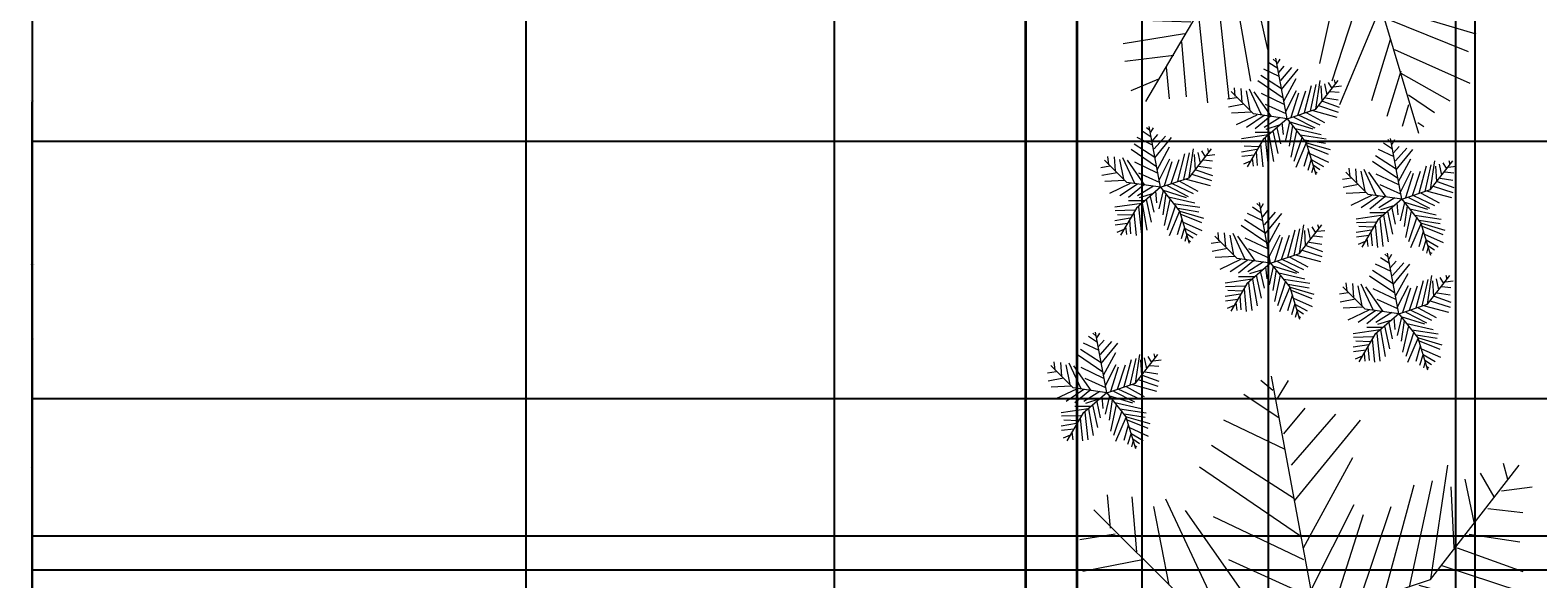
# Model space of a CAD drawing. Units: inches. Extents: x 818 to 1898, y 976 to 2364.
# Tile 60 of 96: x 818 to 1083, y 2046 to 2142. Entities that reach past the tile are written whole.
import ezdxf

# ---------------------------------------------------------------- set-up
doc = ezdxf.new("R2010")
doc.units = ezdxf.units.IN
doc.header["$LTSCALE"] = 5
doc.header["$MEASUREMENT"] = 0
for name, color, linetype, lineweight in [('A-ANNO-DIMS', 2, 'Continuous', 18), ('C-PROP', 7, 'Continuous', 35), ('L-PLNT-BEDS', 94, 'Continuous', 18)]:
    doc.layers.add(name, color=color, linetype=linetype, lineweight=lineweight)
doc.layers.add('L-PLNT', color=116, linetype='Continuous', lineweight=13, true_color=0x136734)
doc.styles.get("Standard").update_dxf_attribs({"font": 'arial.ttf'})
doc.dimstyles.get("Standard").update_dxf_attribs({"dimtxt": 0.18, "dimasz": 0.18, "dimexe": 0.18, "dimexo": 0.0625, "dimgap": 0.09, "dimtad": 0, "dimtih": 1, "dimtoh": 1, "dimdec": 4, "dimzin": 0, "dimdsep": 46, "dimtxsty": 'Standard', "dimcen": 0.09, "dimadec": 0, "dimazin": 0, "dimtfac": 1, "dimtdec": 4, "dimtofl": 0, "dimtmove": 0, "dimatfit": 3, "dimfxl": 1, "dimtolj": 1, "dimtzin": 0, "dimarcsym": 0})

# ---------------------------------------------------------------- blocks, each defined once
blk = doc.blocks.new('SHRUB-ACCENT')
for p, q in [((8.8, 18.63), (7.25, 19.67)), ((8.53, 19.84), (7.99, 20.28)), ((10.44, 9.82), (8.47, 20.47)), ((8.74, 19.5), (9.21, 20.28)), ((9.01, 17.93), (9.96, 19.06)), ((9.35, 16.54), (11.31, 18.8)), ((9.75, 13.42), (5.28, 16.46)), ((9.48, 15.07), (5.82, 17.41)), ((9.08, 17.24), (6.37, 18.54)), ((9.48, 14.98), (12.39, 18.54)), ((9.89, 12.9), (12.06, 16.89)), ((15.49, 11.5), (19.41, 16.55)), ((15.51, 11.51), (16.25, 16.54)), ((17, 15.94), (17.41, 14.03)), ((17.68, 16.2), (18.29, 15.16)), ((18.69, 16.63), (18.9, 15.94)), ((1.56, 13.51), (0, 13.25)), ((4.55, 10.66), (0.62, 14.58)), ((1.35, 13.77), (1.22, 15.24)), ((2.3, 15.16), (2.51, 12.72)), ((3.25, 14.72), (3.93, 11.25)), ((3.79, 15.07), (5.89, 10.55)), ((7.72, 10.21), (4.67, 14.55)), ((5.89, 14.29), (9.89, 12.38)), ((10.23, 11.07), (12.12, 14.81)), ((11.17, 10.12), (12.53, 14.37)), ((12.33, 10.47), (13.75, 14.72)), ((13.48, 10.9), (14.76, 15.68)), ((14.56, 11.16), (15.58, 15.85)), ((16.39, 15.59), (16.53, 12.9)), ((17.2, 13.51), (19.44, 13.16)), ((18.02, 14.63), (19.57, 14.46)), ((18.62, 15.42), (19.98, 15.59)), ((2.84, 12.38), (0.14, 11.86)), ((4.2, 10.99), (0.68, 10.81)), ((10.44, 9.82), (4.55, 10.66)), ((6.57, 12.38), (10.23, 10.73)), ((10.44, 9.82), (15.49, 11.5)), ((13.82, 10.9), (17, 9.16)), ((14.97, 11.25), (19.17, 10.12)), ((15.98, 12.12), (19.44, 10.99)), ((16.66, 12.9), (19.57, 11.86)), ((5.15, 10.47), (1.49, 8.73)), ((6.43, 10.38), (3.32, 8.3)), ((7.45, 10.21), (4.81, 8.04)), ((10.44, 9.82), (6.23, 6.17)), ((9.21, 10.03), (6.43, 8.3)), ((9.21, 8.73), (6.7, 7.95)), ((8.67, 8.21), (9.28, 5.43)), ((9.55, 9.16), (9.75, 7.08)), ((10.9, 9.25), (10.16, 6.04)), ((10.44, 9.82), (13.8, 5.61)), ((10.77, 9.34), (14.97, 8.04)), ((11.38, 8.64), (10.84, 5)), ((11.65, 10.12), (15.31, 8.21)), ((11.85, 8.12), (16.46, 7.08)), ((12.53, 10.47), (16.19, 8.73)), ((7.18, 6.99), (2.44, 6.3)), ((5.89, 5.78), (2.51, 5.69)), ((6.23, 6.17), (3.43, 1.4)), ((7.59, 7.43), (4.81, 7.43)), ((5.76, 5.34), (6.16, 1.35)), ((6.57, 6.39), (7.11, 1.52)), ((7.25, 6.99), (8.06, 2.31)), ((7.92, 7.69), (8.8, 3.69)), ((12.12, 7.69), (11.11, 3.09)), ((13.07, 6.65), (11.65, 2.31)), ((13.82, 5.6), (11.99, 1.26)), ((12.73, 6.99), (17.34, 6.3)), ((13.48, 6.13), (17.2, 5.52)), ((13.8, 5.61), (15.49, 0)), ((13.88, 5.6), (18.02, 4.39)), ((5.15, 4.39), (2.44, 3.95)), ((4.67, 3.43), (2.51, 3.17)), ((5.42, 4.91), (2.91, 5)), ((4.33, 2.91), (4.47, 1.52)), ((5.01, 4.04), (5.21, 1.61)), ((14.22, 4.13), (13.41, 1.44)), ((14.02, 5.08), (17.68, 3.61)), ((14.7, 2.74), (14.09, 0.74)), ((14.43, 3.69), (17.74, 2.22)), ((14.7, 2.65), (16.86, 1.44)), ((4, 2.39), (2.78, 1.87)), ((15.04, 1.26), (14.76, 0.31)), ((15.04, 1.7), (16.19, 0.92)), ((15.44, 0.48), (15.71, 0.31))]:
    blk.add_line(p, q)
blk = doc.blocks.new('PALM-BORDER')
for p, q in [((33.95, 78.95), (31.8, 80.68)), ((41.53, 39.05), (33.72, 81.45)), ((34.76, 77.57), (36.65, 80.68)), ((35.03, 74.11), (28.83, 78.26)), ((35.84, 71.35), (39.61, 75.84)), ((37.18, 65.82), (45, 74.8)), ((36.11, 68.59), (25.33, 73.77)), ((37.72, 59.6), (49.31, 73.77)), ((37.72, 59.95), (23.17, 69.28)), ((39.34, 51.31), (47.96, 67.2)), ((38.8, 53.39), (21.02, 65.48)), ((61.61, 45.75), (77.23, 65.83)), ((61.71, 45.79), (64.67, 65.82)), ((70.33, 64.44), (72.75, 60.3)), ((74.37, 66.17), (75.18, 63.4)), ((53.62, 43.37), (58.74, 62.37)), ((57.93, 44.41), (61.97, 63.06)), ((65.21, 62.02), (65.75, 51.31)), ((67.63, 63.4), (69.25, 55.81)), ((74.1, 61.33), (79.49, 62.02)), ((5.39, 54.77), (4.85, 60.64)), ((9.16, 60.3), (9.97, 50.62)), ((12.93, 58.57), (15.63, 44.75)), ((15.09, 59.95), (23.44, 41.99)), ((40.69, 44.06), (48.23, 58.91)), ((49.04, 41.64), (54.7, 58.57)), ((18.1, 42.4), (2.48, 58.02)), ((30.72, 40.61), (18.59, 57.88)), ((23.44, 56.84), (39.34, 49.24)), ((44.46, 40.26), (49.85, 57.19)), ((71.68, 58.22), (77.87, 57.53)), ((6.2, 53.73), (0, 52.7)), ((68.44, 53.73), (77.33, 52.35)), ((66.29, 51.31), (77.87, 47.17)), ((11.32, 49.24), (0.54, 47.17)), ((26.14, 49.24), (40.69, 42.68)), ((63.59, 48.21), (77.33, 43.71)), ((41.53, 39.05), (61.61, 45.75)), ((16.71, 43.71), (2.69, 43.02)), ((41.53, 39.05), (18.1, 42.4)), ((54.97, 43.37), (67.63, 36.46)), ((59.55, 44.75), (76.26, 40.26)), ((20.48, 41.64), (5.93, 34.73)), ((25.6, 41.3), (13.2, 33.01)), ((29.64, 40.61), (19.13, 31.97)), ((36.65, 39.91), (25.6, 33.01)), ((46.35, 40.26), (60.9, 32.66)), ((49.85, 41.64), (64.4, 34.73)), ((41.53, 39.05), (24.79, 24.55)), ((41.53, 39.05), (54.92, 22.32)), ((42.84, 37.15), (59.55, 31.97)), ((36.65, 34.73), (26.68, 31.62)), ((37.99, 36.46), (38.8, 28.17)), ((43.38, 36.81), (40.42, 24.02)), ((34.49, 32.66), (36.92, 21.61)), ((45.27, 34.39), (43.11, 19.88)), ((47.15, 32.32), (65.48, 28.17)), ((30.18, 29.55), (19.13, 29.55)), ((31.53, 30.59), (35.03, 14.7)), ((48.23, 30.59), (44.19, 12.28)), ((28.56, 27.82), (9.7, 25.06)), ((28.83, 27.82), (32.07, 9.17)), ((50.66, 27.82), (68.98, 25.06)), ((24.79, 24.55), (13.63, 5.58)), ((26.14, 25.41), (28.29, 6.06)), ((52, 26.44), (46.35, 9.17)), ((53.62, 24.37), (68.44, 21.95)), ((23.44, 22.99), (9.97, 22.64)), ((22.9, 21.26), (24.52, 5.37)), ((54.97, 22.3), (47.69, 5.02)), ((54.92, 22.32), (61.61, 0)), ((55.24, 22.3), (71.68, 17.46)), ((21.56, 19.53), (11.59, 19.88)), ((55.78, 20.22), (70.33, 14.35)), ((20.48, 17.46), (9.7, 15.73)), ((19.94, 16.08), (20.75, 6.41)), ((56.59, 16.42), (53.35, 5.72)), ((18.59, 13.66), (9.97, 12.62)), ((57.39, 14.7), (70.6, 8.83)), ((17.24, 11.59), (17.78, 6.06)), ((58.47, 10.9), (56.05, 2.95)), ((15.9, 9.52), (11.05, 7.44)), ((58.47, 10.55), (67.09, 5.72)), ((59.82, 6.75), (64.4, 3.64)), ((59.82, 5.02), (58.74, 1.22)), ((61.44, 1.92), (62.51, 1.22))]:
    blk.add_line(p, q)
blk = doc.blocks.new('PALM-DECK')
for p, q in [((60.66, 141.05), (56.81, 144.14)), ((74.19, 69.77), (60.24, 145.52)), ((62.1, 138.58), (65.47, 144.14)), ((62.58, 132.41), (51.51, 139.82)), ((64.03, 127.47), (70.77, 135.5)), ((66.43, 117.6), (80.4, 133.65)), ((64.51, 122.54), (45.25, 131.79)), ((67.4, 106.49), (88.1, 131.79)), ((67.4, 107.11), (41.4, 123.77)), ((70.29, 91.68), (85.69, 120.07)), ((69.32, 95.38), (37.55, 116.98)), ((110.08, 81.73), (137.98, 117.61)), ((110.24, 81.8), (115.54, 117.6)), ((132.87, 118.22), (134.31, 113.28)), ((125.65, 115.13), (129.98, 107.72)), ((95.8, 77.48), (104.95, 111.43)), ((103.5, 79.33), (110.72, 112.66)), ((120.83, 113.28), (123.72, 99.7)), ((116.5, 110.81), (117.47, 91.68)), ((132.39, 109.58), (142.02, 110.81)), ((9.63, 97.85), (8.67, 108.34)), ((16.37, 107.72), (17.81, 90.44)), ((26.96, 107.11), (41.88, 75.01)), ((32.33, 75.75), (4.43, 103.66)), ((23.11, 104.64), (27.92, 79.95)), ((54.88, 72.55), (33.22, 103.4)), ((72.69, 78.72), (86.17, 105.26)), ((87.62, 74.4), (97.73, 104.64)), ((128.06, 104.02), (139.13, 102.79)), ((41.88, 101.55), (70.29, 87.97)), ((79.43, 71.93), (89.06, 102.17)), ((11.07, 96), (0, 94.15)), ((122.28, 96), (138.16, 93.53)), ((118.43, 91.68), (139.13, 84.27)), ((20.22, 87.97), (0.96, 84.27)), ((46.7, 87.97), (72.69, 76.25)), ((113.61, 86.12), (138.16, 78.1)), ((74.19, 69.77), (110.08, 81.73)), ((106.39, 79.95), (136.24, 71.93)), ((29.85, 78.1), (4.81, 76.87)), ((98.21, 77.48), (120.83, 65.14)), ((36.59, 74.4), (10.59, 62.05)), ((74.19, 69.77), (32.33, 75.75)), ((89.06, 74.4), (115.06, 62.05)), ((45.73, 73.78), (23.59, 58.97)), ((52.96, 72.55), (34.18, 57.12)), ((82.8, 71.93), (108.8, 58.35)), ((74.19, 69.77), (44.29, 43.85)), ((65.47, 71.31), (45.73, 58.97)), ((74.19, 69.77), (98.11, 39.87)), ((76.54, 66.37), (106.39, 57.12)), ((67.88, 65.14), (69.32, 50.33)), ((77.51, 65.76), (72.21, 42.92)), ((65.47, 62.05), (47.66, 56.5)), ((80.88, 61.44), (77.03, 35.52)), ((61.62, 58.35), (65.95, 38.6)), ((84.25, 57.73), (116.98, 50.33)), ((56.33, 54.65), (62.58, 26.26)), ((86.17, 54.65), (78.95, 21.94)), ((53.92, 52.8), (34.18, 52.8)), ((51.03, 49.71), (17.33, 44.77)), ((51.51, 49.71), (57.29, 16.38)), ((90.51, 49.71), (123.24, 44.77)), ((46.7, 45.39), (50.55, 10.83)), ((92.91, 47.24), (82.8, 16.38)), ((44.29, 43.85), (24.36, 9.97)), ((95.8, 43.54), (122.28, 39.22)), ((41.88, 41.07), (17.81, 40.45)), ((98.21, 39.84), (85.21, 8.98)), ((98.11, 39.87), (110.08, 0)), ((98.69, 39.84), (128.06, 31.2)), ((40.92, 37.98), (43.81, 9.59)), ((38.51, 34.9), (20.7, 35.52)), ((99.65, 36.13), (125.65, 25.64)), ((36.59, 31.2), (17.33, 28.11)), ((101.1, 29.34), (95.32, 10.21)), ((35.62, 28.73), (37.07, 11.45)), ((33.22, 24.41), (17.81, 22.55)), ((102.54, 26.26), (126.13, 15.77)), ((30.81, 20.7), (31.77, 10.83)), ((104.47, 19.47), (100.13, 5.27)), ((104.47, 18.85), (119.87, 10.21)), ((28.4, 17), (19.74, 13.3)), ((106.87, 12.06), (115.06, 6.51)), ((106.87, 8.98), (104.95, 2.19)), ((109.76, 3.42), (111.69, 2.19))]:
    blk.add_line(p, q)
blk = doc.blocks.new('*D59')
at = {"layer": 'A-ANNO-DIMS', "color": 0, "lineweight": -2, "ltscale": 5, "transparency": 16777216}
for p, q in [((1251.64, 2300.39), (818.03, 2300.39)), ((818.21, 2300.21), (818.21, 1669.95)), ((818.21, 1039.32), (818.21, 1669.59)), ((896.05, 1039.14), (818.03, 1039.14))]:
    blk.add_line(p, q, dxfattribs=at)
at = {"layer": 'A-ANNO-DIMS', "color": 0, "ltscale": 5, "transparency": 16777216}
for points in [[(818.18, 2300.21), (818.24, 2300.21), (818.21, 2300.39)], [(818.18, 1039.32), (818.24, 1039.32), (818.21, 1039.14)]]:
    blk.add_solid(points, dxfattribs=at)
at = {"layer": 'Defpoints', "color": 0, "ltscale": 5, "transparency": 16777216}
for p in [(818.21, 2300.39), (1251.71, 2300.39), (896.11, 1039.14)]:
    blk.add_point(p, dxfattribs=at)
at = {"layer": 'A-ANNO-DIMS', "color": 0, "ltscale": 5, "transparency": 16777216, "insert": (818.21, 1669.77), "char_height": 0.18, "attachment_point": 5}
blk.add_mtext('\\A1;1261.2', dxfattribs=at)
blk = doc.blocks.new('*D60')
at = {"layer": 'A-ANNO-DIMS', "color": 0, "lineweight": -2, "ltscale": 5, "transparency": 16777216}
for p, q in [((992.66, 2294.22), (818.03, 2294.22)), ((818.21, 2294.04), (818.21, 1748.77)), ((818.21, 1203.14), (818.21, 1748.41)), ((992.66, 1202.96), (818.03, 1202.96))]:
    blk.add_line(p, q, dxfattribs=at)
at = {"layer": 'A-ANNO-DIMS', "color": 0, "ltscale": 5, "transparency": 16777216}
for points in [[(818.18, 2294.04), (818.24, 2294.04), (818.21, 2294.22)], [(818.18, 1203.14), (818.24, 1203.14), (818.21, 1202.96)]]:
    blk.add_solid(points, dxfattribs=at)
at = {"layer": 'Defpoints', "color": 0, "ltscale": 5, "transparency": 16777216}
for p in [(818.21, 2294.22), (992.73, 2294.22), (992.73, 1202.96)]:
    blk.add_point(p, dxfattribs=at)
at = {"layer": 'A-ANNO-DIMS', "color": 0, "ltscale": 5, "transparency": 16777216, "insert": (818.21, 1748.59), "char_height": 0.18, "attachment_point": 5}
blk.add_mtext('\\A1;1091.3', dxfattribs=at)
blk = doc.blocks.new('*D61')
at = {"layer": 'A-ANNO-DIMS', "color": 0, "lineweight": -2, "ltscale": 5, "transparency": 16777216}
for p, q in [((1071.73, 1203.03), (1071.73, 2363.87)), ((1071.91, 2363.69), (1250.94, 2363.69)), ((1430.55, 2363.69), (1251.51, 2363.69)), ((1430.73, 1203.03), (1430.73, 2363.87))]:
    blk.add_line(p, q, dxfattribs=at)
at = {"layer": 'A-ANNO-DIMS', "color": 0, "ltscale": 5, "transparency": 16777216}
for points in [[(1071.91, 2363.72), (1071.91, 2363.66), (1071.73, 2363.69)], [(1430.55, 2363.72), (1430.55, 2363.66), (1430.73, 2363.69)]]:
    blk.add_solid(points, dxfattribs=at)
at = {"layer": 'Defpoints', "color": 0, "ltscale": 5, "transparency": 16777216}
for p in [(1430.73, 2363.69), (1071.73, 1202.96), (1430.73, 1202.96)]:
    blk.add_point(p, dxfattribs=at)
at = {"layer": 'A-ANNO-DIMS', "color": 0, "ltscale": 5, "transparency": 16777216, "insert": (1251.23, 2363.69), "char_height": 0.18, "attachment_point": 5}
blk.add_mtext('\\A1;359', dxfattribs=at)
blk = doc.blocks.new('*D67')
at = {"layer": 'A-ANNO-DIMS', "color": 0, "lineweight": -2, "ltscale": 5, "transparency": 16777216}
for p, q in [((1083.66, 2205.97), (818.03, 2205.97)), ((818.21, 2205.79), (818.21, 2129.71)), ((818.21, 2053.26), (818.21, 2129.34)), ((1083.66, 2053.08), (818.03, 2053.08))]:
    blk.add_line(p, q, dxfattribs=at)
at = {"layer": 'A-ANNO-DIMS', "color": 0, "ltscale": 5, "transparency": 16777216}
for points in [[(818.18, 2205.79), (818.24, 2205.79), (818.21, 2205.97)], [(818.18, 2053.26), (818.24, 2053.26), (818.21, 2053.08)]]:
    blk.add_solid(points, dxfattribs=at)
at = {"layer": 'Defpoints', "color": 0, "ltscale": 5, "transparency": 16777216}
for p in [(818.21, 2205.97), (1083.73, 2205.97), (1083.73, 2053.08)]:
    blk.add_point(p, dxfattribs=at)
at = {"layer": 'A-ANNO-DIMS', "color": 0, "ltscale": 5, "transparency": 16777216, "insert": (818.21, 2129.52), "char_height": 0.18, "attachment_point": 5}
blk.add_mtext('\\A1;152.9', dxfattribs=at)
blk = doc.blocks.new('*D79')
at = {"layer": 'A-ANNO-DIMS', "color": 0, "lineweight": -2, "ltscale": 5, "transparency": 16777216}
for p, q in [((992.73, 1203.03), (992.73, 2363.87)), ((992.91, 2363.69), (1032.01, 2363.69)), ((1071.55, 2363.69), (1032.44, 2363.69)), ((1071.73, 1203.03), (1071.73, 2363.87))]:
    blk.add_line(p, q, dxfattribs=at)
at = {"layer": 'A-ANNO-DIMS', "color": 0, "ltscale": 5, "transparency": 16777216}
for points in [[(992.91, 2363.72), (992.91, 2363.66), (992.73, 2363.69)], [(1071.55, 2363.72), (1071.55, 2363.66), (1071.73, 2363.69)]]:
    blk.add_solid(points, dxfattribs=at)
at = {"layer": 'Defpoints', "color": 0, "ltscale": 5, "transparency": 16777216}
for p in [(1071.73, 2363.69), (992.73, 1202.96), (1071.73, 1202.96)]:
    blk.add_point(p, dxfattribs=at)
at = {"layer": 'A-ANNO-DIMS', "color": 0, "ltscale": 5, "transparency": 16777216, "insert": (1032.23, 2363.69), "char_height": 0.18, "attachment_point": 5}
blk.add_mtext('\\A1;79', dxfattribs=at)
blk = doc.blocks.new('*D90')
at = {"layer": 'A-ANNO-DIMS', "color": 0, "lineweight": -2, "ltscale": 5, "transparency": 16777216}
for p, q in [((904.95, 1071.12), (904.95, 2363.87)), ((905.13, 2363.69), (931.67, 2363.69)), ((958.99, 2363.69), (932.45, 2363.69)), ((959.17, 1071.12), (959.17, 2363.87))]:
    blk.add_line(p, q, dxfattribs=at)
at = {"layer": 'A-ANNO-DIMS', "color": 0, "ltscale": 5, "transparency": 16777216}
for points in [[(905.13, 2363.72), (905.13, 2363.66), (904.95, 2363.69)], [(958.99, 2363.72), (958.99, 2363.66), (959.17, 2363.69)]]:
    blk.add_solid(points, dxfattribs=at)
at = {"layer": 'Defpoints', "color": 0, "ltscale": 5, "transparency": 16777216}
for p in [(959.17, 2363.69), (904.95, 1071.06), (959.17, 1071.06)]:
    blk.add_point(p, dxfattribs=at)
at = {"layer": 'A-ANNO-DIMS', "color": 0, "ltscale": 5, "transparency": 16777216, "insert": (932.06, 2363.69), "char_height": 0.18, "attachment_point": 5}
blk.add_mtext('\\A1;54.22', dxfattribs=at)
blk = doc.blocks.new('*D91')
at = {"layer": 'A-ANNO-DIMS', "color": 0, "lineweight": -2, "ltscale": 5, "transparency": 16777216}
for p, q in [((959.17, 1071.12), (959.17, 2363.87)), ((959.35, 2363.69), (985.8, 2363.69)), ((1013.04, 2363.69), (986.59, 2363.69)), ((1013.22, 1071.12), (1013.22, 2363.87))]:
    blk.add_line(p, q, dxfattribs=at)
at = {"layer": 'A-ANNO-DIMS', "color": 0, "ltscale": 5, "transparency": 16777216}
for points in [[(959.35, 2363.72), (959.35, 2363.66), (959.17, 2363.69)], [(1013.04, 2363.72), (1013.04, 2363.66), (1013.22, 2363.69)]]:
    blk.add_solid(points, dxfattribs=at)
at = {"layer": 'Defpoints', "color": 0, "ltscale": 5, "transparency": 16777216}
for p in [(1013.22, 2363.69), (959.17, 1071.06), (1013.22, 1071.06)]:
    blk.add_point(p, dxfattribs=at)
at = {"layer": 'A-ANNO-DIMS', "color": 0, "ltscale": 5, "transparency": 16777216, "insert": (986.2, 2363.69), "char_height": 0.18, "attachment_point": 5}
blk.add_mtext('\\A1;54.04', dxfattribs=at)
blk = doc.blocks.new('*D92')
at = {"layer": 'A-ANNO-DIMS', "color": 0, "lineweight": -2, "ltscale": 5, "transparency": 16777216}
for p, q in [((1013.22, 1071.12), (1013.22, 2363.87)), ((1013.4, 2363.69), (1040.38, 2363.69)), ((1068.16, 2363.69), (1041.17, 2363.69)), ((1068.34, 1071.12), (1068.34, 2363.87))]:
    blk.add_line(p, q, dxfattribs=at)
at = {"layer": 'A-ANNO-DIMS', "color": 0, "ltscale": 5, "transparency": 16777216}
for points in [[(1013.4, 2363.72), (1013.4, 2363.66), (1013.22, 2363.69)], [(1068.16, 2363.72), (1068.16, 2363.66), (1068.34, 2363.69)]]:
    blk.add_solid(points, dxfattribs=at)
at = {"layer": 'Defpoints', "color": 0, "ltscale": 5, "transparency": 16777216}
for p in [(1068.34, 2363.69), (1013.22, 1071.06), (1068.34, 1071.06)]:
    blk.add_point(p, dxfattribs=at)
at = {"layer": 'A-ANNO-DIMS', "color": 0, "ltscale": 5, "transparency": 16777216, "insert": (1040.78, 2363.69), "char_height": 0.18, "attachment_point": 5}
blk.add_mtext('\\A1;55.12', dxfattribs=at)
blk = doc.blocks.new('*D93')
at = {"layer": 'A-ANNO-DIMS', "color": 0, "lineweight": -2, "ltscale": 5, "transparency": 16777216}
for p, q in [((1068.34, 1071.12), (1068.34, 2363.87)), ((1068.52, 2363.69), (1094.16, 2363.69)), ((1120.58, 2363.69), (1094.94, 2363.69)), ((1120.76, 1071.12), (1120.76, 2363.87))]:
    blk.add_line(p, q, dxfattribs=at)
at = {"layer": 'A-ANNO-DIMS', "color": 0, "ltscale": 5, "transparency": 16777216}
for points in [[(1068.52, 2363.72), (1068.52, 2363.66), (1068.34, 2363.69)], [(1120.58, 2363.72), (1120.58, 2363.66), (1120.76, 2363.69)]]:
    blk.add_solid(points, dxfattribs=at)
at = {"layer": 'Defpoints', "color": 0, "ltscale": 5, "transparency": 16777216}
for p in [(1120.76, 2363.69), (1068.34, 1071.06), (1120.76, 1071.06)]:
    blk.add_point(p, dxfattribs=at)
at = {"layer": 'A-ANNO-DIMS', "color": 0, "ltscale": 5, "transparency": 16777216, "insert": (1094.55, 2363.69), "char_height": 0.18, "attachment_point": 5}
blk.add_mtext('\\A1;52.42', dxfattribs=at)
blk = doc.blocks.new('*D126')
at = {"layer": 'A-ANNO-DIMS', "color": 0, "lineweight": -2, "ltscale": 5, "transparency": 16777216}
for p, q in [((1035.38, 1252.09), (1035.38, 2363.87)), ((1035.56, 2363.69), (1075.41, 2363.69)), ((1116.01, 2363.69), (1076.16, 2363.69)), ((1116.19, 1236.03), (1116.19, 2363.87))]:
    blk.add_line(p, q, dxfattribs=at)
at = {"layer": 'A-ANNO-DIMS', "color": 0, "ltscale": 5, "transparency": 16777216}
for points in [[(1035.56, 2363.72), (1035.56, 2363.66), (1035.38, 2363.69)], [(1116.01, 2363.72), (1116.01, 2363.66), (1116.19, 2363.69)]]:
    blk.add_solid(points, dxfattribs=at)
at = {"layer": 'Defpoints', "color": 0, "ltscale": 5, "transparency": 16777216}
for p in [(1035.38, 2363.69), (1035.38, 1252.02), (1116.19, 1235.96)]:
    blk.add_point(p, dxfattribs=at)
at = {"layer": 'A-ANNO-DIMS', "color": 0, "ltscale": 5, "transparency": 16777216, "insert": (1075.78, 2363.69), "char_height": 0.18, "attachment_point": 5}
blk.add_mtext('\\A1;80.81', dxfattribs=at)
blk = doc.blocks.new('*D133')
at = {"layer": 'A-ANNO-DIMS', "color": 0, "lineweight": -2, "ltscale": 5, "transparency": 16777216}
for p, q in [((1041.64, 2162.89), (818.03, 2162.89)), ((818.21, 2162.71), (818.21, 2101.01)), ((818.21, 2038.94), (818.21, 2100.64)), ((1043.71, 2038.76), (818.03, 2038.76))]:
    blk.add_line(p, q, dxfattribs=at)
at = {"layer": 'A-ANNO-DIMS', "color": 0, "ltscale": 5, "transparency": 16777216}
for points in [[(818.18, 2162.71), (818.24, 2162.71), (818.21, 2162.89)], [(818.18, 2038.94), (818.24, 2038.94), (818.21, 2038.76)]]:
    blk.add_solid(points, dxfattribs=at)
at = {"layer": 'Defpoints', "color": 0, "ltscale": 5, "transparency": 16777216}
for p in [(818.21, 2162.89), (1041.7, 2162.89), (1043.77, 2038.76)]:
    blk.add_point(p, dxfattribs=at)
at = {"layer": 'A-ANNO-DIMS', "color": 0, "ltscale": 5, "transparency": 16777216, "insert": (818.21, 2100.82), "char_height": 0.18, "attachment_point": 5}
blk.add_mtext('\\A1;124.13', dxfattribs=at)
blk = doc.blocks.new('*D146')
at = {"layer": 'A-ANNO-DIMS', "color": 0, "lineweight": -2, "ltscale": 5, "transparency": 16777216}
for p, q in [((1197.33, 2122.38), (818.03, 2122.38)), ((818.21, 2122.2), (818.21, 2087.91)), ((818.21, 2053.26), (818.21, 2087.55)), ((1083.66, 2053.08), (818.03, 2053.08))]:
    blk.add_line(p, q, dxfattribs=at)
at = {"layer": 'A-ANNO-DIMS', "color": 0, "ltscale": 5, "transparency": 16777216}
for points in [[(818.18, 2122.2), (818.24, 2122.2), (818.21, 2122.38)], [(818.18, 2053.26), (818.24, 2053.26), (818.21, 2053.08)]]:
    blk.add_solid(points, dxfattribs=at)
at = {"layer": 'Defpoints', "color": 0, "ltscale": 5, "transparency": 16777216}
for p in [(1197.39, 2122.38), (818.21, 2053.08), (1083.73, 2053.08)]:
    blk.add_point(p, dxfattribs=at)
at = {"layer": 'A-ANNO-DIMS', "color": 0, "ltscale": 5, "transparency": 16777216, "insert": (818.21, 2087.73), "char_height": 0.18, "attachment_point": 5}
blk.add_mtext('\\A1;69.3', dxfattribs=at)
blk = doc.blocks.new('*D257')
at = {"layer": 'A-ANNO-DIMS', "color": 0, "lineweight": -2, "ltscale": 5, "transparency": 16777216}
for p, q in [((1399.57, 2077.19), (818.03, 2077.19)), ((818.21, 2077.01), (818.21, 2065.31)), ((818.21, 2053.26), (818.21, 2064.95)), ((1399.57, 2053.08), (818.03, 2053.08))]:
    blk.add_line(p, q, dxfattribs=at)
at = {"layer": 'A-ANNO-DIMS', "color": 0, "ltscale": 5, "transparency": 16777216}
for points in [[(818.18, 2077.01), (818.24, 2077.01), (818.21, 2077.19)], [(818.18, 2053.26), (818.24, 2053.26), (818.21, 2053.08)]]:
    blk.add_solid(points, dxfattribs=at)
at = {"layer": 'Defpoints', "color": 0, "ltscale": 5, "transparency": 16777216}
for p in [(818.21, 2077.19), (1399.64, 2077.19), (1399.64, 2053.08)]:
    blk.add_point(p, dxfattribs=at)
at = {"layer": 'A-ANNO-DIMS', "color": 0, "ltscale": 5, "transparency": 16777216, "insert": (818.21, 2065.13), "char_height": 0.18, "attachment_point": 5}
blk.add_mtext('\\A1;24.11', dxfattribs=at)
blk = doc.blocks.new('*D266')
at = {"layer": 'A-ANNO-DIMS', "color": 0, "lineweight": -2, "ltscale": 5, "transparency": 16777216}
for p, q in [((1780.44, 2053.08), (818.03, 2053.08)), ((818.21, 2052.9), (818.21, 2050.26)), ((818.21, 2047.26), (818.21, 2049.9)), ((1780.44, 2047.08), (818.03, 2047.08))]:
    blk.add_line(p, q, dxfattribs=at)
at = {"layer": 'A-ANNO-DIMS', "color": 0, "ltscale": 5, "transparency": 16777216}
for points in [[(818.18, 2052.9), (818.24, 2052.9), (818.21, 2053.08)], [(818.18, 2047.26), (818.24, 2047.26), (818.21, 2047.08)]]:
    blk.add_solid(points, dxfattribs=at)
at = {"layer": 'Defpoints', "color": 0, "ltscale": 5, "transparency": 16777216}
for p in [(1780.5, 2053.08), (818.21, 2047.08), (1780.5, 2047.08)]:
    blk.add_point(p, dxfattribs=at)
at = {"layer": 'A-ANNO-DIMS', "color": 0, "ltscale": 5, "transparency": 16777216, "insert": (818.21, 2050.08), "char_height": 0.18, "attachment_point": 5}
blk.add_mtext('\\A1;6', dxfattribs=at)

msp = doc.modelspace()

# ---------------------------------------------------------------- linework, layer by layer
at = {"layer": 'C-PROP'}
for p, q in [((992.7251, 2294.2171), (992.7251, 1202.9642)), ((1001.7252, 2285.2171), (1001.7252, 1211.9642))]:
    msp.add_line(p, q, dxfattribs=at)
at = {"layer": 'L-PLNT-BEDS'}
msp.add_line((1071.7251, 2214.9709), (1071.7251, 1202.9642), dxfattribs=at)

# ---------------------------------------------------------------- block references
at = {"layer": 'L-PLNT'}
for name, p in [('PALM-BORDER', (1000.173, 2123.8387)), ('SHRUB-ACCENT', (1028.2232, 2116.571)), ('SHRUB-ACCENT', (1005.9728, 2104.5394)), ('SHRUB-ACCENT', (1048.3795, 2102.447)), ('SHRUB-ACCENT', (1025.3438, 2091.2001)), ('SHRUB-ACCENT', (1047.856, 2082.3073)), ('SHRUB-ACCENT', (996.5491, 2068.4448)), ('PALM-BORDER', (1002.2407, 1999.7071)), ('PALM-DECK', (1057.571, 1904.8049))]:
    msp.add_blockref(name, p, dxfattribs=at)

# ---------------------------------------------------------------- dimensions: what is measured, and where the dimension line sits
at = {"layer": 'A-ANNO-DIMS', "ltscale": 5}
for base, p1, p2, override, picture, middle in [((959.1737, 2363.6929), (904.9504, 1071.0552), (959.1737, 1071.0552), {"dimdec": 2, "dimlfac": 1, "dimrnd": 0, "dimzin": 0, "dimdsep": 46, "dimlunit": 2}, '*D90', (932.062, 2363.6929)), ((1013.2176, 2363.6929), (959.1737, 1071.0552), (1013.2176, 1071.0552), {"dimdec": 2, "dimlfac": 1, "dimrnd": 0, "dimzin": 0, "dimdsep": 46, "dimlunit": 2}, '*D91', (986.1956, 2363.6929)), ((1071.7251, 2363.6929), (992.7251, 1202.9642), (1071.7251, 1202.9642), {"dimdec": 0, "dimlfac": 1, "dimrnd": 0, "dimzin": 0, "dimdsep": 46, "dimlunit": 2}, '*D79', (1032.2251, 2363.6929)), ((1068.3377, 2363.6929), (1013.2176, 1071.0552), (1068.3377, 1071.0552), {"dimdec": 2, "dimlfac": 1, "dimrnd": 0, "dimzin": 0, "dimdsep": 46, "dimlunit": 2}, '*D92', (1040.7776, 2363.6929)), ((1035.3768, 2363.6929), (1116.1882, 1235.9642), (1035.3768, 1252.0242), {"dimdec": 2, "dimlfac": 1, "dimrnd": 0, "dimzin": 0, "dimdsep": 46, "dimlunit": 2}, '*D126', (1075.7825, 2363.6929)), ((1120.7618, 2363.6929), (1068.3377, 1071.0552), (1120.7618, 1071.0552), {"dimdec": 2, "dimlfac": 1, "dimrnd": 0, "dimzin": 0, "dimdsep": 46, "dimlunit": 2}, '*D93', (1094.5497, 2363.6929)), ((1430.7251, 2363.6929), (1071.7251, 1202.9642), (1430.7251, 1202.9642), {"dimdec": 0, "dimlfac": 1, "dimrnd": 0, "dimzin": 0, "dimdsep": 46, "dimlunit": 2}, '*D61', (1251.2251, 2363.6929))]:
    dim = msp.add_linear_dim(base=base, p1=p1, p2=p2, dimstyle='Standard', override=override, dxfattribs=at)
    dim.commit()
    dim.dimension.update_dxf_attribs({"geometry": picture, "text_midpoint": middle})
for base, p1, p2, override, picture, middle in [((818.2059, 2300.3929), (896.1138, 1039.1433), (1251.7057, 2300.3929), {"dimdec": 1, "dimlfac": 1, "dimrnd": 0, "dimzin": 0, "dimdsep": 46, "dimlunit": 2}, '*D59', (818.2059, 1669.7681)), ((818.2059, 2294.2171), (992.7251, 1202.9642), (992.7251, 2294.2171), {"dimdec": 1, "dimlfac": 1, "dimrnd": 0, "dimzin": 0, "dimdsep": 46, "dimlunit": 2}, '*D60', (818.2059, 1748.5907)), ((818.2059, 2205.9709), (1083.7251, 2053.0782), (1083.7251, 2205.9709), {"dimdec": 1, "dimlfac": 1, "dimrnd": 0, "dimzin": 0, "dimdsep": 46, "dimlunit": 2}, '*D67', (818.2059, 2129.5246)), ((818.2059, 2162.8898), (1043.7685, 2038.7583), (1041.7008, 2162.8898), {"dimdec": 2, "dimlfac": 1, "dimrnd": 0, "dimzin": 0, "dimdsep": 46, "dimlunit": 2}, '*D133', (818.2059, 2100.824)), ((818.2059, 2053.0782), (1197.3925, 2122.3767), (1083.7251, 2053.0782), {"dimdec": 1, "dimlfac": 1, "dimrnd": 0, "dimzin": 0, "dimdsep": 46, "dimlunit": 2}, '*D146', (818.2059, 2087.7275)), ((818.2059, 2077.1881), (1399.6356, 2053.0782), (1399.6356, 2077.1881), {"dimdec": 2, "dimlfac": 1, "dimrnd": 0, "dimzin": 0, "dimdsep": 46, "dimlunit": 2}, '*D257', (818.2059, 2065.1332)), ((818.2059, 2047.0782), (1780.5019, 2053.0782), (1780.5019, 2047.0782), {"dimdec": 0, "dimlfac": 1, "dimrnd": 0, "dimzin": 0, "dimdsep": 46, "dimlunit": 2}, '*D266', (818.2059, 2050.0782))]:
    dim = msp.add_linear_dim(base=base, p1=p1, p2=p2, angle=90, dimstyle='Standard', override=override, dxfattribs=at)
    dim.commit()
    dim.dimension.update_dxf_attribs({"geometry": picture, "text_midpoint": middle})

doc.saveas('drawing.dxf')
